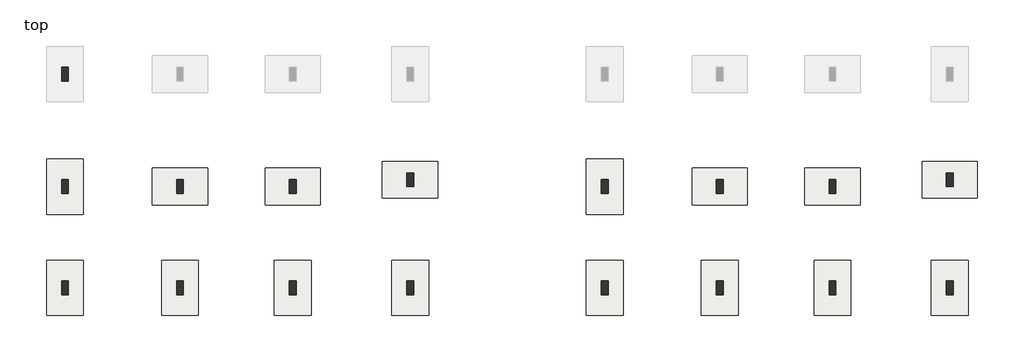
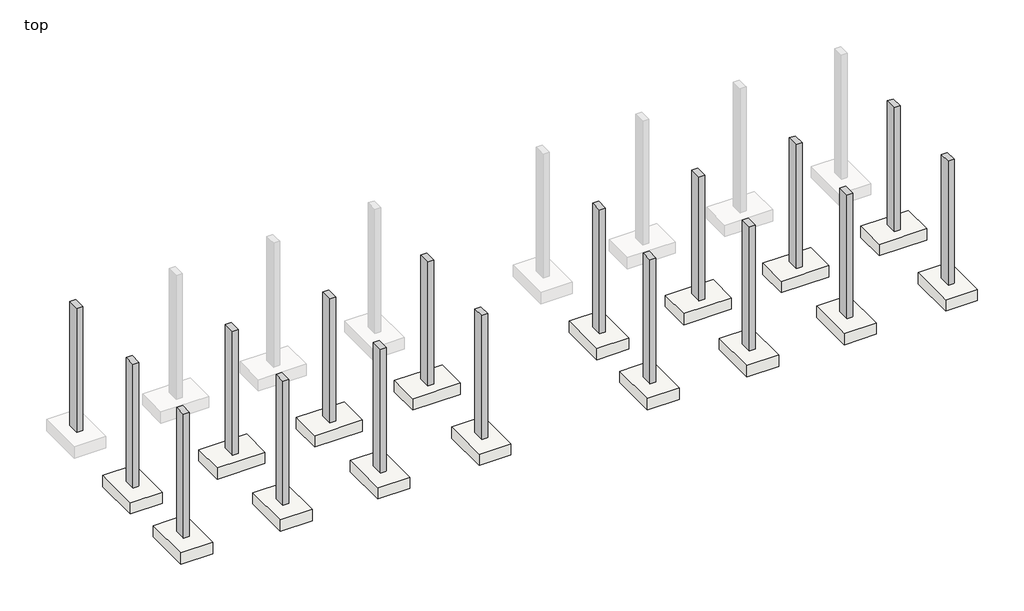
# One storey, part 1 of 2: 17 columns, 16 slabs.
"""IFC4 building model written with IfcOpenShell, lengths in millimetres."""

from ifc_helpers import new_model, si_unit, frame, origin, place, context, project, spatial, polyline, outline, extrude, faceted_brep, element, save

model = new_model("IFC4")

# Units and contexts
model_context = context("Model", 3, world=origin())
ifc_project = project(units=[si_unit("LENGTHUNIT", "METRE", prefix="MILLI")], contexts=[model_context])

# Site, building, storey
site = spatial("IfcSite", under=ifc_project)
building = spatial("IfcBuilding", under=site)
storey = spatial("IfcBuildingStorey", under=building, Name="top", Elevation=-1219.2)

# Columns
placement = place(None, origin())
element("IfcColumn", 1, ObjectType="Concrete-Rectangular-Column", at=placement, inside=storey, context=model_context, shape_type="Brep", body=[
    faceted_brep([(-16071.9993763, 2938.4935985, -1219.2), (-16071.9993763, 2481.2935985, -1219.2), (-16300.5993763, 2481.2935985, -1219.2), (-16300.5993763, 2938.4935985, -1219.2), (-16071.9993763, 2938.4935985, 3810.0), (-16071.9993763, 2481.2935985, 3810.0), (-16071.9993763, 2481.2935985, 3200.4), (-16071.9993763, 2481.2935985, 609.6), (-16071.9993763, 2481.2935985, 0.0), (-16071.9993763, 2938.4935985, 0.0), (-16071.9993763, 2938.4935985, 609.6), (-16071.9993763, 2938.4935985, 3200.4), (-16300.5993763, 2481.2935985, 3810.0), (-16300.5993763, 2481.2935985, 3200.4), (-16300.5993763, 2481.2935985, 609.6), (-16300.5993763, 2481.2935985, 0.0), (-16300.5993763, 2938.4935985, 3810.0), (-16300.5993763, 2938.4935985, 3200.4), (-16300.5993763, 2938.4935985, 609.6), (-16300.5993763, 2938.4935985, 0.0)], [[[0, 1, 2, 3]], [[4, 5, 6, 7, 8, 1, 0, 9, 10, 11]], [[5, 12, 13, 14, 15, 2, 1, 8, 7, 6]], [[12, 16, 17, 18, 19, 3, 2, 15, 14, 13]], [[16, 4, 11, 10, 9, 0, 3, 19, 18, 17]], [[4, 16, 12, 5]]]),
])
element("IfcColumn", 2, ObjectType="Concrete-Rectangular-Column", at=placement, inside=storey, context=model_context, shape_type="Brep", body=[
    faceted_brep([(-4641.9993763, -566.7064015, -1219.2), (-4641.9993763, -1023.9064015, -1219.2), (-4870.5993763, -1023.9064015, -1219.2), (-4870.5993763, -566.7064015, -1219.2), (-4641.9993763, -566.7064015, 3810.0), (-4641.9993763, -1023.9064015, 3810.0), (-4641.9993763, -1023.9064015, 3200.4), (-4641.9993763, -1023.9064015, 609.6), (-4641.9993763, -1023.9064015, 0.0), (-4641.9993763, -566.7064015, 0.0), (-4641.9993763, -566.7064015, 609.6), (-4641.9993763, -566.7064015, 3200.4), (-4870.5993763, -1023.9064015, 3810.0), (-4870.5993763, -1023.9064015, 3200.4), (-4870.5993763, -1023.9064015, 609.6), (-4870.5993763, -1023.9064015, 0.0), (-4870.5993763, -566.7064015, 3810.0), (-4870.5993763, -566.7064015, 3200.4), (-4870.5993763, -566.7064015, 609.6), (-4870.5993763, -566.7064015, 0.0)], [[[0, 1, 2, 3]], [[4, 5, 6, 7, 8, 1, 0, 9, 10, 11]], [[5, 12, 13, 14, 15, 2, 1, 8, 7, 6]], [[12, 16, 17, 18, 19, 3, 2, 15, 14, 13]], [[16, 4, 11, 10, 9, 0, 3, 19, 18, 17]], [[4, 16, 12, 5]]]),
])
element("IfcColumn", 3, ObjectType="Concrete-Rectangular-Column", at=placement, inside=storey, context=model_context, shape_type="Brep", body=[
    faceted_brep([(-12261.9993763, -795.3064015, -1219.2), (-12261.9993763, -1252.5064015, -1219.2), (-12490.5993763, -1252.5064015, -1219.2), (-12490.5993763, -795.3064015, -1219.2), (-12261.9993763, -795.3064015, 3810.0), (-12261.9993763, -1023.9064015, 3810.0), (-12261.9993763, -1252.5064015, 3810.0), (-12261.9993763, -1252.5064015, 3200.4), (-12261.9993763, -1252.5064015, 609.6), (-12261.9993763, -1252.5064015, 0.0), (-12261.9993763, -795.3064015, 0.0), (-12261.9993763, -795.3064015, 609.6), (-12261.9993763, -795.3064015, 3200.4), (-12490.5993763, -1252.5064015, 3810.0), (-12490.5993763, -1252.5064015, 3200.4), (-12490.5993763, -1252.5064015, 609.6), (-12490.5993763, -1252.5064015, 0.0), (-12490.5993763, -1023.9064015, 3810.0), (-12490.5993763, -795.3064015, 3810.0), (-12490.5993763, -795.3064015, 3200.4), (-12490.5993763, -795.3064015, 609.6), (-12490.5993763, -795.3064015, 0.0)], [[[0, 1, 2, 3]], [[4, 5, 6, 7, 8, 9, 1, 0, 10, 11, 12]], [[6, 13, 14, 15, 16, 2, 1, 9, 8, 7]], [[13, 17, 18, 19, 20, 21, 3, 2, 16, 15, 14]], [[18, 4, 12, 11, 10, 0, 3, 21, 20, 19]], [[4, 18, 17, 13, 6, 5]]]),
])
element("IfcColumn", 4, ObjectType="Concrete-Rectangular-Column", at=placement, inside=storey, context=model_context, shape_type="Brep", body=[
    faceted_brep([(-16071.9993763, -795.3064015, -1219.2), (-16071.9993763, -1252.5064015, -1219.2), (-16300.5993763, -1252.5064015, -1219.2), (-16300.5993763, -795.3064015, -1219.2), (-16071.9993763, -795.3064015, 3810.0), (-16071.9993763, -1252.5064015, 3810.0), (-16071.9993763, -1252.5064015, 3200.4), (-16071.9993763, -1252.5064015, 609.6), (-16071.9993763, -1252.5064015, 0.0), (-16071.9993763, -795.3064015, 0.0), (-16071.9993763, -795.3064015, 609.6), (-16071.9993763, -795.3064015, 3200.4), (-16300.5993763, -1252.5064015, 3810.0), (-16300.5993763, -1252.5064015, 3200.4), (-16300.5993763, -1252.5064015, 609.6), (-16300.5993763, -1252.5064015, 0.0), (-16300.5993763, -795.3064015, 3810.0), (-16300.5993763, -795.3064015, 3200.4), (-16300.5993763, -795.3064015, 609.6), (-16300.5993763, -795.3064015, 0.0)], [[[0, 1, 2, 3]], [[4, 5, 6, 7, 8, 1, 0, 9, 10, 11]], [[5, 12, 13, 14, 15, 2, 1, 8, 7, 6]], [[12, 16, 17, 18, 19, 3, 2, 15, 14, 13]], [[16, 4, 11, 10, 9, 0, 3, 19, 18, 17]], [[4, 16, 12, 5]]]),
])
element("IfcColumn", 5, ObjectType="Concrete-Rectangular-Column", at=placement, inside=storey, context=model_context, shape_type="Brep", body=[
    faceted_brep([(-16071.9993763, -4148.1064015, -1219.2), (-16071.9993763, -4605.3064015, -1219.2), (-16300.5993763, -4605.3064015, -1219.2), (-16300.5993763, -4148.1064015, -1219.2), (-16071.9993763, -4148.1064015, 3810.0), (-16071.9993763, -4605.3064015, 3810.0), (-16071.9993763, -4148.1064015, 0.0), (-16071.9993763, -4148.1064015, 609.6), (-16300.5993763, -4605.3064015, 3810.0), (-16300.5993763, -4148.1064015, 3810.0), (-16300.5993763, -4148.1064015, 609.6), (-16300.5993763, -4148.1064015, 0.0)], [[[0, 1, 2, 3]], [[4, 5, 1, 0, 6, 7]], [[5, 8, 2, 1]], [[8, 9, 10, 11, 3, 2]], [[9, 4, 7, 6, 0, 3, 11, 10]], [[4, 9, 8, 5]]]),
])
element("IfcColumn", 6, ObjectType="Concrete-Rectangular-Column", at=placement, inside=storey, context=model_context, shape_type="Brep", body=[
    faceted_brep([(-12261.9993763, -4148.1064015, -1219.2), (-12261.9993763, -4605.3064015, -1219.2), (-12490.5993763, -4605.3064015, -1219.2), (-12490.5993763, -4148.1064015, -1219.2), (-12261.9993763, -4148.1064015, 3810.0), (-12261.9993763, -4605.3064015, 3810.0), (-12261.9993763, -4148.1064015, 0.0), (-12261.9993763, -4148.1064015, 609.6), (-12490.5993763, -4605.3064015, 3810.0), (-12490.5993763, -4605.3064015, 609.6), (-12490.5993763, -4605.3064015, 0.0), (-12490.5993763, -4148.1064015, 3810.0), (-12490.5993763, -4148.1064015, 609.6), (-12490.5993763, -4148.1064015, 0.0)], [[[0, 1, 2, 3]], [[4, 5, 1, 0, 6, 7]], [[5, 8, 9, 10, 2, 1]], [[8, 11, 12, 13, 3, 2, 10, 9]], [[11, 4, 7, 6, 0, 3, 13, 12]], [[4, 11, 8, 5]]]),
])
element("IfcColumn", 7, ObjectType="Concrete-Rectangular-Column", at=placement, inside=storey, context=model_context, shape_type="Brep", body=[
    faceted_brep([(-8528.1993763, -4148.1064015, -1219.2), (-8528.1993763, -4605.3064015, -1219.2), (-8756.7993763, -4605.3064015, -1219.2), (-8756.7993763, -4148.1064015, -1219.2), (-8528.1993763, -4148.1064015, 3810.0), (-8528.1993763, -4605.3064015, 3810.0), (-8528.1993763, -4605.3064015, 3200.4), (-8528.1993763, -4605.3064015, 609.6), (-8528.1993763, -4605.3064015, 0.0), (-8528.1993763, -4148.1064015, 0.0), (-8528.1993763, -4148.1064015, 609.6), (-8528.1993763, -4148.1064015, 3200.4), (-8756.7993763, -4605.3064015, 3810.0), (-8756.7993763, -4605.3064015, 3200.4), (-8756.7993763, -4605.3064015, 609.6), (-8756.7993763, -4605.3064015, 0.0), (-8756.7993763, -4148.1064015, 3810.0), (-8756.7993763, -4148.1064015, 3200.4), (-8756.7993763, -4148.1064015, 609.6), (-8756.7993763, -4148.1064015, 0.0)], [[[0, 1, 2, 3]], [[4, 5, 6, 7, 8, 1, 0, 9, 10, 11]], [[5, 12, 13, 14, 15, 2, 1, 8, 7, 6]], [[12, 16, 17, 18, 19, 3, 2, 15, 14, 13]], [[16, 4, 11, 10, 9, 0, 3, 19, 18, 17]], [[4, 16, 12, 5]]]),
])
element("IfcColumn", 8, ObjectType="Concrete-Rectangular-Column", at=placement, inside=storey, context=model_context, shape_type="Brep", body=[
    faceted_brep([(-4641.9993763, -4148.1064015, -1219.2), (-4641.9993763, -4605.3064015, -1219.2), (-4870.5993763, -4605.3064015, -1219.2), (-4870.5993763, -4148.1064015, -1219.2), (-4641.9993763, -4148.1064015, 3810.0), (-4641.9993763, -4605.3064015, 3810.0), (-4641.9993763, -4148.1064015, 0.0), (-4641.9993763, -4148.1064015, 609.6), (-4870.5993763, -4605.3064015, 3810.0), (-4870.5993763, -4605.3064015, 609.6), (-4870.5993763, -4605.3064015, 0.0), (-4870.5993763, -4148.1064015, 3810.0), (-4870.5993763, -4148.1064015, 609.6), (-4870.5993763, -4148.1064015, 0.0)], [[[0, 1, 2, 3]], [[4, 5, 1, 0, 6, 7]], [[5, 8, 9, 10, 2, 1]], [[8, 11, 12, 13, 3, 2, 10, 9]], [[11, 4, 7, 6, 0, 3, 13, 12]], [[4, 11, 8, 5]]]),
])
element("IfcColumn", 9, ObjectType="Concrete-Rectangular-Column", at=placement, inside=storey, context=model_context, shape_type="Brep", body=[
    faceted_brep([(-8528.1993763, -795.3064015, -1219.2), (-8528.1993763, -1252.5064015, -1219.2), (-8756.7993763, -1252.5064015, -1219.2), (-8756.7993763, -795.3064015, -1219.2), (-8528.1993763, -795.3064015, 3810.0), (-8528.1993763, -1252.5064015, 3810.0), (-8528.1993763, -1252.5064015, 3200.4), (-8528.1993763, -1252.5064015, 609.6), (-8528.1993763, -1252.5064015, 0.0), (-8528.1993763, -795.3064015, 0.0), (-8528.1993763, -795.3064015, 609.6), (-8528.1993763, -795.3064015, 3200.4), (-8756.7993763, -1252.5064015, 3810.0), (-8756.7993763, -1252.5064015, 3200.4), (-8756.7993763, -1252.5064015, 609.6), (-8756.7993763, -1252.5064015, 0.0), (-8756.7993763, -795.3064015, 3810.0), (-8756.7993763, -795.3064015, 3200.4), (-8756.7993763, -795.3064015, 609.6), (-8756.7993763, -795.3064015, 0.0)], [[[0, 1, 2, 3]], [[4, 5, 6, 7, 8, 1, 0, 9, 10, 11]], [[5, 12, 13, 14, 15, 2, 1, 8, 7, 6]], [[12, 16, 17, 18, 19, 3, 2, 15, 14, 13]], [[16, 4, 11, 10, 9, 0, 3, 19, 18, 17]], [[4, 16, 12, 5]]]),
])
element("IfcColumn", 10, ObjectType="Concrete-Rectangular-Column", at=placement, inside=storey, context=model_context, shape_type="Brep", body=[
    faceted_brep([(13232.5761273, -566.7064015, -1219.2), (13232.5761273, -1023.9064015, -1219.2), (13003.9761273, -1023.9064015, -1219.2), (13003.9761273, -566.7064015, -1219.2), (13232.5761273, -566.7064015, 3810.0), (13232.5761273, -1023.9064015, 3810.0), (13232.5761273, -1023.9064015, 3200.4), (13232.5761273, -1023.9064015, 609.6), (13232.5761273, -1023.9064015, 0.0), (13232.5761273, -566.7064015, 0.0), (13232.5761273, -566.7064015, 609.6), (13232.5761273, -566.7064015, 3200.4), (13003.9761273, -1023.9064015, 3810.0), (13003.9761273, -1023.9064015, 3200.4), (13003.9761273, -1023.9064015, 609.6), (13003.9761273, -1023.9064015, 0.0), (13003.9761273, -566.7064015, 3810.0), (13003.9761273, -566.7064015, 3200.4), (13003.9761273, -566.7064015, 609.6), (13003.9761273, -566.7064015, 0.0)], [[[0, 1, 2, 3]], [[4, 5, 6, 7, 8, 1, 0, 9, 10, 11]], [[5, 12, 13, 14, 15, 2, 1, 8, 7, 6]], [[12, 16, 17, 18, 19, 3, 2, 15, 14, 13]], [[16, 4, 11, 10, 9, 0, 3, 19, 18, 17]], [[4, 16, 12, 5]]]),
])
element("IfcColumn", 11, ObjectType="Concrete-Rectangular-Column", at=placement, inside=storey, context=model_context, shape_type="Brep", body=[
    faceted_brep([(5612.5761273, -795.3064015, -1219.2), (5612.5761273, -1252.5064015, -1219.2), (5383.9761273, -1252.5064015, -1219.2), (5383.9761273, -795.3064015, -1219.2), (5612.5761273, -795.3064015, 3810.0), (5612.5761273, -1023.9064015, 3810.0), (5612.5761273, -1252.5064015, 3810.0), (5612.5761273, -1252.5064015, 3200.4), (5612.5761273, -1252.5064015, 609.6), (5612.5761273, -1252.5064015, 0.0), (5612.5761273, -795.3064015, 0.0), (5612.5761273, -795.3064015, 609.6), (5612.5761273, -795.3064015, 3200.4), (5383.9761273, -1252.5064015, 3810.0), (5383.9761273, -1252.5064015, 3200.4), (5383.9761273, -1252.5064015, 609.6), (5383.9761273, -1252.5064015, 0.0), (5383.9761273, -1023.9064015, 3810.0), (5383.9761273, -795.3064015, 3810.0), (5383.9761273, -795.3064015, 3200.4), (5383.9761273, -795.3064015, 609.6), (5383.9761273, -795.3064015, 0.0)], [[[0, 1, 2, 3]], [[4, 5, 6, 7, 8, 9, 1, 0, 10, 11, 12]], [[6, 13, 14, 15, 16, 2, 1, 9, 8, 7]], [[13, 17, 18, 19, 20, 21, 3, 2, 16, 15, 14]], [[18, 4, 12, 11, 10, 0, 3, 21, 20, 19]], [[4, 18, 17, 13, 6, 5]]]),
])
element("IfcColumn", 12, ObjectType="Concrete-Rectangular-Column", at=placement, inside=storey, context=model_context, shape_type="Brep", body=[
    faceted_brep([(1802.5761273, -795.3064015, -1219.2), (1802.5761273, -1252.5064015, -1219.2), (1573.9761273, -1252.5064015, -1219.2), (1573.9761273, -795.3064015, -1219.2), (1802.5761273, -795.3064015, 3810.0), (1802.5761273, -1252.5064015, 3810.0), (1802.5761273, -1252.5064015, 3200.4), (1802.5761273, -1252.5064015, 609.6), (1802.5761273, -1252.5064015, 0.0), (1802.5761273, -795.3064015, 0.0), (1802.5761273, -795.3064015, 609.6), (1802.5761273, -795.3064015, 3200.4), (1573.9761273, -1252.5064015, 3810.0), (1573.9761273, -1252.5064015, 3200.4), (1573.9761273, -1252.5064015, 609.6), (1573.9761273, -1252.5064015, 0.0), (1573.9761273, -795.3064015, 3810.0), (1573.9761273, -795.3064015, 3200.4), (1573.9761273, -795.3064015, 609.6), (1573.9761273, -795.3064015, 0.0)], [[[0, 1, 2, 3]], [[4, 5, 6, 7, 8, 1, 0, 9, 10, 11]], [[5, 12, 13, 14, 15, 2, 1, 8, 7, 6]], [[12, 16, 17, 18, 19, 3, 2, 15, 14, 13]], [[16, 4, 11, 10, 9, 0, 3, 19, 18, 17]], [[4, 16, 12, 5]]]),
])
element("IfcColumn", 13, ObjectType="Concrete-Rectangular-Column", at=placement, inside=storey, context=model_context, shape_type="Brep", body=[
    faceted_brep([(1802.5761273, -4148.1064015, -1219.2), (1802.5761273, -4605.3064015, -1219.2), (1573.9761273, -4605.3064015, -1219.2), (1573.9761273, -4148.1064015, -1219.2), (1802.5761273, -4148.1064015, 3810.0), (1802.5761273, -4605.3064015, 3810.0), (1802.5761273, -4148.1064015, 0.0), (1802.5761273, -4148.1064015, 609.6), (1573.9761273, -4605.3064015, 3810.0), (1573.9761273, -4148.1064015, 3810.0), (1573.9761273, -4148.1064015, 609.6), (1573.9761273, -4148.1064015, 0.0)], [[[0, 1, 2, 3]], [[4, 5, 1, 0, 6, 7]], [[5, 8, 2, 1]], [[8, 9, 10, 11, 3, 2]], [[9, 4, 7, 6, 0, 3, 11, 10]], [[4, 9, 8, 5]]]),
])
element("IfcColumn", 14, ObjectType="Concrete-Rectangular-Column", at=placement, inside=storey, context=model_context, shape_type="Brep", body=[
    faceted_brep([(5612.5761273, -4148.1064015, -1219.2), (5612.5761273, -4605.3064015, -1219.2), (5383.9761273, -4605.3064015, -1219.2), (5383.9761273, -4148.1064015, -1219.2), (5612.5761273, -4148.1064015, 3810.0), (5612.5761273, -4605.3064015, 3810.0), (5612.5761273, -4148.1064015, 0.0), (5612.5761273, -4148.1064015, 609.6), (5383.9761273, -4605.3064015, 3810.0), (5383.9761273, -4605.3064015, 609.6), (5383.9761273, -4605.3064015, 0.0), (5383.9761273, -4148.1064015, 3810.0), (5383.9761273, -4148.1064015, 609.6), (5383.9761273, -4148.1064015, 0.0)], [[[0, 1, 2, 3]], [[4, 5, 1, 0, 6, 7]], [[5, 8, 9, 10, 2, 1]], [[8, 11, 12, 13, 3, 2, 10, 9]], [[11, 4, 7, 6, 0, 3, 13, 12]], [[4, 11, 8, 5]]]),
])
element("IfcColumn", 15, ObjectType="Concrete-Rectangular-Column", at=placement, inside=storey, context=model_context, shape_type="Brep", body=[
    faceted_brep([(9346.3761273, -4148.1064015, -1219.2), (9346.3761273, -4605.3064015, -1219.2), (9117.7761273, -4605.3064015, -1219.2), (9117.7761273, -4148.1064015, -1219.2), (9346.3761273, -4148.1064015, 3810.0), (9346.3761273, -4605.3064015, 3810.0), (9346.3761273, -4605.3064015, 3200.4), (9346.3761273, -4605.3064015, 609.6), (9346.3761273, -4605.3064015, 0.0), (9346.3761273, -4148.1064015, 0.0), (9346.3761273, -4148.1064015, 609.6), (9346.3761273, -4148.1064015, 3200.4), (9117.7761273, -4605.3064015, 3810.0), (9117.7761273, -4605.3064015, 3200.4), (9117.7761273, -4605.3064015, 609.6), (9117.7761273, -4605.3064015, 0.0), (9117.7761273, -4148.1064015, 3810.0), (9117.7761273, -4148.1064015, 3200.4), (9117.7761273, -4148.1064015, 609.6), (9117.7761273, -4148.1064015, 0.0)], [[[0, 1, 2, 3]], [[4, 5, 6, 7, 8, 1, 0, 9, 10, 11]], [[5, 12, 13, 14, 15, 2, 1, 8, 7, 6]], [[12, 16, 17, 18, 19, 3, 2, 15, 14, 13]], [[16, 4, 11, 10, 9, 0, 3, 19, 18, 17]], [[4, 16, 12, 5]]]),
])
element("IfcColumn", 16, ObjectType="Concrete-Rectangular-Column", at=placement, inside=storey, context=model_context, shape_type="Brep", body=[
    faceted_brep([(13232.5761273, -4148.1064015, -1219.2), (13232.5761273, -4605.3064015, -1219.2), (13003.9761273, -4605.3064015, -1219.2), (13003.9761273, -4148.1064015, -1219.2), (13232.5761273, -4148.1064015, 3810.0), (13232.5761273, -4605.3064015, 3810.0), (13232.5761273, -4148.1064015, 0.0), (13232.5761273, -4148.1064015, 609.6), (13003.9761273, -4605.3064015, 3810.0), (13003.9761273, -4605.3064015, 609.6), (13003.9761273, -4605.3064015, 0.0), (13003.9761273, -4148.1064015, 3810.0), (13003.9761273, -4148.1064015, 609.6), (13003.9761273, -4148.1064015, 0.0)], [[[0, 1, 2, 3]], [[4, 5, 1, 0, 6, 7]], [[5, 8, 9, 10, 2, 1]], [[8, 11, 12, 13, 3, 2, 10, 9]], [[11, 4, 7, 6, 0, 3, 13, 12]], [[4, 11, 8, 5]]]),
])
element("IfcColumn", 17, ObjectType="Concrete-Rectangular-Column", at=placement, inside=storey, context=model_context, shape_type="Brep", body=[
    faceted_brep([(9346.3761273, -795.3064015, -1219.2), (9346.3761273, -1252.5064015, -1219.2), (9117.7761273, -1252.5064015, -1219.2), (9117.7761273, -795.3064015, -1219.2), (9346.3761273, -795.3064015, 3810.0), (9346.3761273, -1252.5064015, 3810.0), (9346.3761273, -1252.5064015, 3200.4), (9346.3761273, -1252.5064015, 609.6), (9346.3761273, -1252.5064015, 0.0), (9346.3761273, -795.3064015, 0.0), (9346.3761273, -795.3064015, 609.6), (9346.3761273, -795.3064015, 3200.4), (9117.7761273, -1252.5064015, 3810.0), (9117.7761273, -1252.5064015, 3200.4), (9117.7761273, -1252.5064015, 609.6), (9117.7761273, -1252.5064015, 0.0), (9117.7761273, -795.3064015, 3810.0), (9117.7761273, -795.3064015, 3200.4), (9117.7761273, -795.3064015, 609.6), (9117.7761273, -795.3064015, 0.0)], [[[0, 1, 2, 3]], [[4, 5, 6, 7, 8, 1, 0, 9, 10, 11]], [[5, 12, 13, 14, 15, 2, 1, 8, 7, 6]], [[12, 16, 17, 18, 19, 3, 2, 15, 14, 13]], [[16, 4, 11, 10, 9, 0, 3, 19, 18, 17]], [[4, 16, 12, 5]]]),
])

# Slabs
element("IfcSlab", 18, ObjectType="Footing-Rectangular : 72\" x 48\" x 18\"", at=placement, inside=storey, context=model_context, shape_type="SweptSolid", body=[
    extrude(outline(polyline([(-5670.6993763, -185.7064015), (-3841.8993763, -185.7064015), (-3841.8993763, -1404.9064015), (-5670.6993763, -1404.9064015), (-5670.6993763, -185.7064015)])), frame((0.0, 0.0, -1676.4), z_axis=(0.0, 0.0, 1.0), x_axis=(1.0, 0.0, 0.0)), (0.0, 0.0, 1.0), 457.2),
])
element("IfcSlab", 19, ObjectType="Footing-Rectangular : 72\" x 48\" x 18\"", at=placement, inside=storey, context=model_context, shape_type="SweptSolid", body=[
    extrude(outline(polyline([(-13290.6993763, -414.3064015), (-11461.8993763, -414.3064015), (-11461.8993763, -1633.5064015), (-13290.6993763, -1633.5064015), (-13290.6993763, -414.3064015)])), frame((0.0, 0.0, -1676.4), z_axis=(0.0, 0.0, 1.0), x_axis=(1.0, 0.0, 0.0)), (0.0, 0.0, 1.0), 457.2),
])
element("IfcSlab", 20, ObjectType="Footing-Rectangular : 72\" x 48\" x 18\"", at=placement, inside=storey, context=model_context, shape_type="SweptSolid", body=[
    extrude(outline(polyline([(-15576.6993763, -109.5064015), (-15576.6993763, -1938.3064015), (-16795.8993763, -1938.3064015), (-16795.8993763, -109.5064015), (-15576.6993763, -109.5064015)])), frame((0.0, 0.0, -1676.4), z_axis=(0.0, 0.0, 1.0), x_axis=(1.0, 0.0, 0.0)), (0.0, 0.0, 1.0), 457.2),
])
element("IfcSlab", 21, ObjectType="Footing-Rectangular : 72\" x 48\" x 18\"", at=placement, inside=storey, context=model_context, shape_type="SweptSolid", body=[
    extrude(outline(polyline([(-15576.6993763, -3462.3064015), (-15576.6993763, -5291.1064015), (-16795.8993763, -5291.1064015), (-16795.8993763, -3462.3064015), (-15576.6993763, -3462.3064015)])), frame((0.0, 0.0, -1676.4), z_axis=(0.0, 0.0, 1.0), x_axis=(1.0, 0.0, 0.0)), (0.0, 0.0, 1.0), 457.2),
])
element("IfcSlab", 22, ObjectType="Footing-Rectangular : 72\" x 48\" x 18\"", at=placement, inside=storey, context=model_context, shape_type="SweptSolid", body=[
    extrude(outline(polyline([(-11766.6993763, -3462.3064015), (-11766.6993763, -5291.1064015), (-12985.8993763, -5291.1064015), (-12985.8993763, -3462.3064015), (-11766.6993763, -3462.3064015)])), frame((0.0, 0.0, -1676.4), z_axis=(0.0, 0.0, 1.0), x_axis=(1.0, 0.0, 0.0)), (0.0, 0.0, 1.0), 457.2),
])
element("IfcSlab", 23, ObjectType="Footing-Rectangular : 72\" x 48\" x 18\"", at=placement, inside=storey, context=model_context, shape_type="SweptSolid", body=[
    extrude(outline(polyline([(-8032.8993763, -3462.3064015), (-8032.8993763, -5291.1064015), (-9252.0993763, -5291.1064015), (-9252.0993763, -3462.3064015), (-8032.8993763, -3462.3064015)])), frame((0.0, 0.0, -1676.4), z_axis=(0.0, 0.0, 1.0), x_axis=(1.0, 0.0, 0.0)), (0.0, 0.0, 1.0), 457.2),
])
element("IfcSlab", 24, ObjectType="Footing-Rectangular : 72\" x 48\" x 18\"", at=placement, inside=storey, context=model_context, shape_type="SweptSolid", body=[
    extrude(outline(polyline([(-4146.6993763, -3462.3064015), (-4146.6993763, -5291.1064015), (-5365.8993763, -5291.1064015), (-5365.8993763, -3462.3064015), (-4146.6993763, -3462.3064015)])), frame((0.0, 0.0, -1676.4), z_axis=(0.0, 0.0, 1.0), x_axis=(1.0, 0.0, 0.0)), (0.0, 0.0, 1.0), 457.2),
])
element("IfcSlab", 25, ObjectType="Footing-Rectangular : 72\" x 48\" x 18\"", at=placement, inside=storey, context=model_context, shape_type="SweptSolid", body=[
    extrude(outline(polyline([(-9556.8993763, -414.3064015), (-7728.0993763, -414.3064015), (-7728.0993763, -1633.5064015), (-9556.8993763, -1633.5064015), (-9556.8993763, -414.3064015)])), frame((0.0, 0.0, -1676.4), z_axis=(0.0, 0.0, 1.0), x_axis=(1.0, 0.0, 0.0)), (0.0, 0.0, 1.0), 457.2),
])
element("IfcSlab", 26, ObjectType="Footing-Rectangular : 72\" x 48\" x 18\"", at=placement, inside=storey, context=model_context, shape_type="SweptSolid", body=[
    extrude(outline(polyline([(12203.8761273, -185.7064015), (14032.6761273, -185.7064015), (14032.6761273, -1404.9064015), (12203.8761273, -1404.9064015), (12203.8761273, -185.7064015)])), frame((0.0, 0.0, -1676.4), z_axis=(0.0, 0.0, 1.0), x_axis=(1.0, 0.0, 0.0)), (0.0, 0.0, 1.0), 457.2),
])
element("IfcSlab", 27, ObjectType="Footing-Rectangular : 72\" x 48\" x 18\"", at=placement, inside=storey, context=model_context, shape_type="SweptSolid", body=[
    extrude(outline(polyline([(4583.8761273, -414.3064015), (6412.6761273, -414.3064015), (6412.6761273, -1633.5064015), (4583.8761273, -1633.5064015), (4583.8761273, -414.3064015)])), frame((0.0, 0.0, -1676.4), z_axis=(0.0, 0.0, 1.0), x_axis=(1.0, 0.0, 0.0)), (0.0, 0.0, 1.0), 457.2),
])
element("IfcSlab", 28, ObjectType="Footing-Rectangular : 72\" x 48\" x 18\"", at=placement, inside=storey, context=model_context, shape_type="SweptSolid", body=[
    extrude(outline(polyline([(2297.8761273, -109.5064015), (2297.8761273, -1938.3064015), (1078.6761273, -1938.3064015), (1078.6761273, -109.5064015), (2297.8761273, -109.5064015)])), frame((0.0, 0.0, -1676.4), z_axis=(0.0, 0.0, 1.0), x_axis=(1.0, 0.0, 0.0)), (0.0, 0.0, 1.0), 457.2),
])
element("IfcSlab", 29, ObjectType="Footing-Rectangular : 72\" x 48\" x 18\"", at=placement, inside=storey, context=model_context, shape_type="SweptSolid", body=[
    extrude(outline(polyline([(2297.8761273, -3462.3064015), (2297.8761273, -5291.1064015), (1078.6761273, -5291.1064015), (1078.6761273, -3462.3064015), (2297.8761273, -3462.3064015)])), frame((0.0, 0.0, -1676.4), z_axis=(0.0, 0.0, 1.0), x_axis=(1.0, 0.0, 0.0)), (0.0, 0.0, 1.0), 457.2),
])
element("IfcSlab", 30, ObjectType="Footing-Rectangular : 72\" x 48\" x 18\"", at=placement, inside=storey, context=model_context, shape_type="SweptSolid", body=[
    extrude(outline(polyline([(6107.8761273, -3462.3064015), (6107.8761273, -5291.1064015), (4888.6761273, -5291.1064015), (4888.6761273, -3462.3064015), (6107.8761273, -3462.3064015)])), frame((0.0, 0.0, -1676.4), z_axis=(0.0, 0.0, 1.0), x_axis=(1.0, 0.0, 0.0)), (0.0, 0.0, 1.0), 457.2),
])
element("IfcSlab", 31, ObjectType="Footing-Rectangular : 72\" x 48\" x 18\"", at=placement, inside=storey, context=model_context, shape_type="SweptSolid", body=[
    extrude(outline(polyline([(9841.6761273, -3462.3064015), (9841.6761273, -5291.1064015), (8622.4761273, -5291.1064015), (8622.4761273, -3462.3064015), (9841.6761273, -3462.3064015)])), frame((0.0, 0.0, -1676.4), z_axis=(0.0, 0.0, 1.0), x_axis=(1.0, 0.0, 0.0)), (0.0, 0.0, 1.0), 457.2),
])
element("IfcSlab", 32, ObjectType="Footing-Rectangular : 72\" x 48\" x 18\"", at=placement, inside=storey, context=model_context, shape_type="SweptSolid", body=[
    extrude(outline(polyline([(13727.8761273, -3462.3064015), (13727.8761273, -5291.1064015), (12508.6761273, -5291.1064015), (12508.6761273, -3462.3064015), (13727.8761273, -3462.3064015)])), frame((0.0, 0.0, -1676.4), z_axis=(0.0, 0.0, 1.0), x_axis=(1.0, 0.0, 0.0)), (0.0, 0.0, 1.0), 457.2),
])
element("IfcSlab", 33, ObjectType="Footing-Rectangular : 72\" x 48\" x 18\"", at=placement, inside=storey, context=model_context, shape_type="SweptSolid", body=[
    extrude(outline(polyline([(8317.6761273, -414.3064015), (10146.4761273, -414.3064015), (10146.4761273, -1633.5064015), (8317.6761273, -1633.5064015), (8317.6761273, -414.3064015)])), frame((0.0, 0.0, -1676.4), z_axis=(0.0, 0.0, 1.0), x_axis=(1.0, 0.0, 0.0)), (0.0, 0.0, 1.0), 457.2),
])

save(model, "model.ifc")

# Revit data of these elements
# Type "Concrete-Rectangular-Column"
#   Assembly Code = "B10"
#   b = 0' - 9"
#   h = 1' - 6"
#   Structural Material [instance default] = Concrete, Cast-in-Place gray
# Type "Footing-Rectangular : 72\" x 48\" x 18\""
#   Assembly Code = "A1010100"
#   Width = 4' - 0"
#   Length = 6' - 0"
#   Foundation Thickness = 1' - 6"
#   Structural Material [instance default] = Concrete, Cast-in-Place gray
# Elements 1, 2, 3, 4, 5, 6, 7, 8, 9, 10, 11, 12, 13, 14, 15, 16, 17 (IfcColumn, "Concrete-Rectangular-Column")
#   Structural Material = Concrete, Cast-in-Place gray
#   Phase Created = New Construction
#   Materials on its faces: "Concrete, Cast-in-Place gray"
# Elements 18, 19, 20, 21, 22, 23, 24, 25, 26, 27, 28, 29, 30, 31, 32, 33 (IfcSlab, "Footing-Rectangular : 72\" x 48\" x 18\"")
#   Structural Material = Concrete, Cast-in-Place gray
#   Phase Created = New Construction
#   Materials on its faces: "Concrete, Cast-in-Place gray"
# Materials
#   "Concrete, Cast-in-Place gray": class "Concrete", colour RGB 192 192 192, transparency 0, Description = "Cast-in-place concrete", Cost = 0
